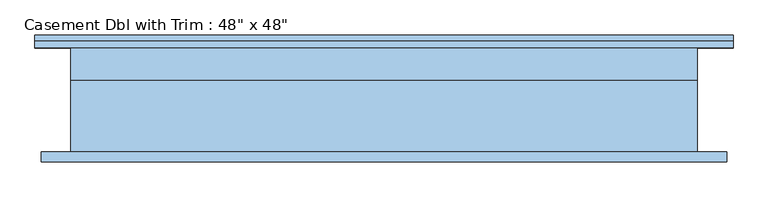
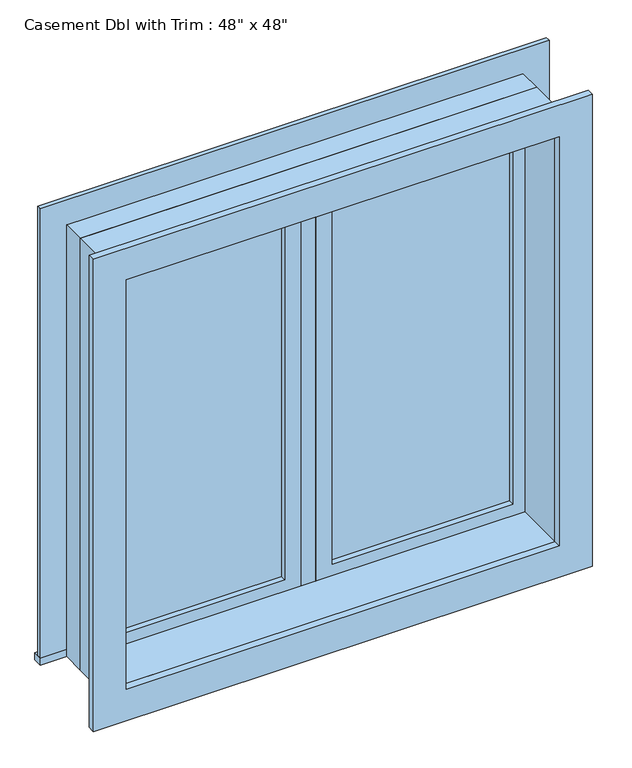
"""IFC4 building model written with IfcOpenShell, lengths in millimetres: window geometry."""

from ifc_helpers import new_model, si_unit, frame, origin, place, context, project, spatial, polyline, outline, extrude, source, transform, mapped, element, save


def window_0862ab64(model_context):
    return source(origin(), model_context, "Body", "SweptSolid", [
        extrude(outline(polyline([(63.5, 85.725), (546.1, 85.725), (546.1, 73.025), (63.5, 73.025), (63.5, 85.725)])), frame((0.0, 0.0, 977.9), z_axis=(0.0, 0.0, 1.0), x_axis=(1.0, 0.0, 0.0)), (0.0, 0.0, 1.0), 1092.2),
        extrude(outline(polyline([(2114.55, 19.05), (933.45, 19.05), (933.45, 590.55), (2114.55, 590.55), (2114.55, 19.05)]), holes=[polyline([(2070.1, 63.5), (2070.1, 546.1), (977.9, 546.1), (977.9, 63.5), (2070.1, 63.5)])]), frame((0.0, 57.15, 0.0), z_axis=(0.0, 1.0, 0.0), x_axis=(0.0, 0.0, 1.0)), (0.0, 0.0, 1.0), 44.45),
        extrude(outline(polyline([(19.05, 57.15), (-19.05, 57.15), (-19.05, 120.65), (19.05, 120.65), (19.05, 57.15)])), frame((0.0, 0.0, 933.45), z_axis=(0.0, 0.0, 1.0), x_axis=(1.0, 0.0, 0.0)), (0.0, 0.0, 1.0), 1181.1),
        extrude(outline(polyline([(-679.45, 146.05), (679.45, 146.05), (679.45, 120.65), (-679.45, 120.65), (-679.45, 146.05)])), frame((0.0, 0.0, 914.4), z_axis=(0.0, 0.0, 1.0), x_axis=(1.0, 0.0, 0.0)), (0.0, 0.0, 1.0), 19.05),
        extrude(outline(polyline([(2114.55, -590.55), (2114.55, 590.55), (933.45, 590.55), (933.45, 679.45), (2203.45, 679.45), (2203.45, -679.45), (933.45, -679.45), (933.45, -590.55), (2114.55, -590.55)])), frame((0.0, 120.65, 0.0), z_axis=(0.0, 1.0, 0.0), x_axis=(0.0, 0.0, 1.0)), (0.0, 0.0, 1.0), 12.7),
        extrude(outline(polyline([(2190.75, 666.75), (2190.75, -666.75), (857.25, -666.75), (857.25, 666.75), (2190.75, 666.75)]), holes=[polyline([(2101.85, 577.85), (946.15, 577.85), (946.15, -577.85), (2101.85, -577.85), (2101.85, 577.85)])]), frame((0.0, -101.6, 0.0), z_axis=(0.0, 1.0, 0.0), x_axis=(0.0, 0.0, 1.0)), (0.0, 0.0, 1.0), 19.05),
        extrude(outline(polyline([(-63.5, 73.025), (-546.1, 73.025), (-546.1, 85.725), (-63.5, 85.725), (-63.5, 73.025)])), frame((0.0, 0.0, 977.9), z_axis=(0.0, 0.0, 1.0), x_axis=(1.0, 0.0, 0.0)), (0.0, 0.0, 1.0), 1092.2),
        extrude(outline(polyline([(2114.55, -590.55), (933.45, -590.55), (933.45, -19.05), (2114.55, -19.05), (2114.55, -590.55)]), holes=[polyline([(2070.1, -546.1), (2070.1, -63.5), (977.9, -63.5), (977.9, -546.1), (2070.1, -546.1)])]), frame((0.0, 57.15, 0.0), z_axis=(0.0, 1.0, 0.0), x_axis=(0.0, 0.0, 1.0)), (0.0, 0.0, 1.0), 44.45),
        extrude(outline(polyline([(2133.6, -609.6), (914.4, -609.6), (914.4, 609.6), (2133.6, 609.6), (2133.6, -609.6)]), holes=[polyline([(2101.85, -577.85), (2101.85, 577.85), (946.15, 577.85), (946.15, -577.85), (2101.85, -577.85)])]), frame((0.0, -82.55, 0.0), z_axis=(0.0, 1.0, 0.0), x_axis=(0.0, 0.0, 1.0)), (0.0, 0.0, 1.0), 139.7),
        extrude(outline(polyline([(2133.6, 609.6), (2133.6, -609.6), (914.4, -609.6), (914.4, 609.6), (2133.6, 609.6)]), holes=[polyline([(2114.55, 590.55), (933.45, 590.55), (933.45, -590.55), (2114.55, -590.55), (2114.55, 590.55)])]), frame((0.0, 57.15, 0.0), z_axis=(0.0, 1.0, 0.0), x_axis=(0.0, 0.0, 1.0)), (0.0, 0.0, 1.0), 63.5),
    ])


if __name__ == "__main__":
    model = new_model("IFC4")
    model_context = context("Model", 3, world=origin())
    ifc_project = project(units=[si_unit("LENGTHUNIT", "METRE", prefix="MILLI")], contexts=[model_context])
    site = spatial("IfcSite", under=ifc_project)
    building = spatial("IfcBuilding", under=site)
    placement = place(None, origin())
    window_shape = window_0862ab64(model_context)
    element("IfcWindow", 1, ObjectType="Casement Dbl with Trim : 48\" x 48\"", at=placement, inside=building, context=model_context, shape_type="MappedRepresentation", body=[
        mapped(window_shape, transform((0.0, 0.0, 0.0), x_axis=(1.0, 0.0, 0.0), y_axis=(0.0, 1.0, 0.0), z_axis=(0.0, 0.0, 1.0))),
    ])
    save(model, "model.ifc")

# Revit data of these elements
# Type "Casement Dbl with Trim : 48\" x 48\""
#   Type Mark = "32"
#   Construction Type Id = "GSP4R"
#   Assembly Code = "B2020100"
#   Analytic Construction = "1/8 in Pilkington single glazing"
#   Visual Light Transmittance = 0.9
#   Solar Heat Gain Coefficient = 0.78
#   Heat Transfer Coefficient (U) = 0.6496 BTU/(h·ft²·°F)
#   Height = 4' - 0"
#   Default Sill Height = 3' - 0"
#   Trim Projection - Ext. = 0' - 0 1/2"
#   Trim Projection - Int. = 0' - 0 3/4"
#   Trim Width - Exterior = 0' - 3 1/2"
#   Trim Width - Interior = 0' - 3 1/2"
#   Width = 4' - 0"
#   Window Inset = 0' - 0 3/4"
#   Define Thermal Properties by = 1
#   Glass Pane Material = Glass
#   Sash Material = Sash
#   Trim Exterior Material = Trim
#   Trim Interior Material = Trim
#   Wall Closure = (empty or 0)
# Element 1 (IfcWindow, "Casement Dbl with Trim : 48\" x 48\"")
#   Materials on its faces: "Sash", "Trim", "Glass"
# Materials
#   "Glass": class "Glass", colour RGB 0 128 192, transparency 0.75, Description = "Soda Lime Glass", Cost = 0
#   "Sash": class "Wood", colour RGB 224 178 126, transparency 0
#   "Trim": class "Wood", colour RGB 224 178 126, transparency 0
